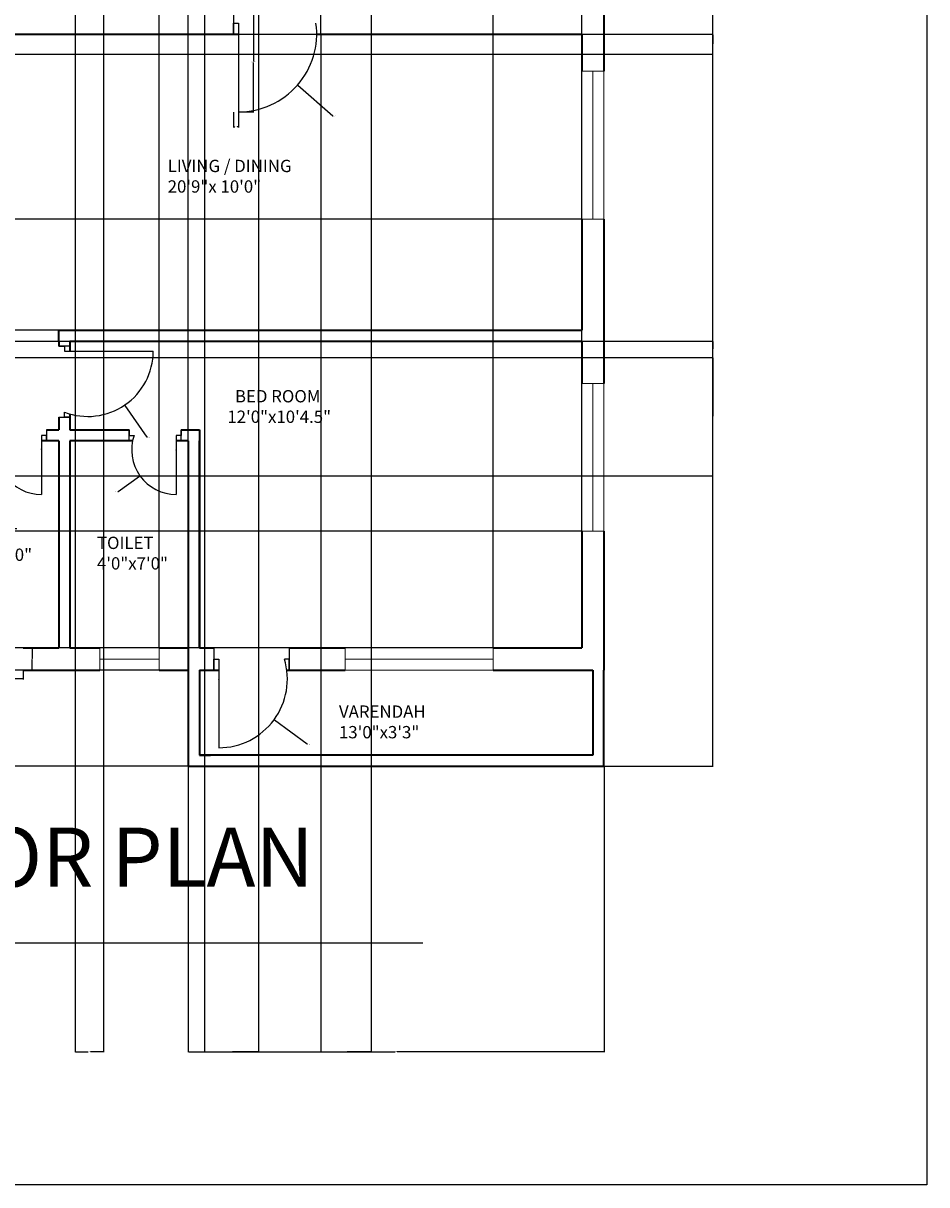
# Model space of a CAD drawing. Units: inches. Extents: x 1870 to 2611, y 1432 to 2511.
# Tile 2 of 5: x 2245 to 2611, y 1432 to 1903. Entities that reach past the tile are written whole.
import ezdxf

# ---------------------------------------------------------------- set-up
doc = ezdxf.new("R2010")
doc.units = ezdxf.units.IN
for name, color, linetype, lineweight in [('A-ANNO-DIMS', 2, 'Continuous', 18), ('A-ANNO-TTLB', 7, 'Continuous', 25), ('A-AREA-IDEN', 7, 'Continuous', 18), ('A-DOOR', 31, 'Continuous', 25), ('A-GLAZ', 201, 'Continuous', 18), ('A-WALL', 7, 'Continuous', 35)]:
    doc.layers.add(name, color=color, linetype=linetype, lineweight=lineweight)
doc.styles.get("Standard").update_dxf_attribs({"font": 'arial.ttf'})
doc.dimstyles.get("Standard").update_dxf_attribs({"dimtxt": 0.18, "dimasz": 0.18, "dimexe": 0.18, "dimexo": 0.0625, "dimgap": 0.09, "dimtad": 0, "dimtih": 1, "dimtoh": 1, "dimdec": 4, "dimzin": 0, "dimdsep": 46, "dimtxsty": 'Standard', "dimcen": 0.09, "dimadec": 0, "dimazin": 0, "dimtfac": 1, "dimtdec": 4, "dimtofl": 0, "dimtmove": 0, "dimatfit": 3, "dimfxl": 1, "dimtolj": 1, "dimtzin": 0, "dimarcsym": 0})

# ---------------------------------------------------------------- blocks, each defined once
blk = doc.blocks.new('DOOR-LEAF-36-JAMB-4P5')
for p, q in [((36, 2), (0, 2)), ((33.75, 0), (38.25, 0)), ((36, 0), (36, 2)), ((38.25, 0), (36, 0))]:
    blk.add_line(p, q)
blk = doc.blocks.new('DOOR-LEAF-24-JAMB-4P5')
for p, q in [((2, 2.25), (2, 26.25)), ((0, 4.5), (0, 0)), ((0, 0), (0, 2.25)), ((0, 2.25), (2, 2.25))]:
    blk.add_line(p, q)
blk = doc.blocks.new('DOOR-LEAF-36-JAMB-9-B')
for p, q in [((0, 40.5), (0, 31.5)), ((0, 31.5), (0, 36)), ((0, 36), (2, 36)), ((2, 36), (2, 0))]:
    blk.add_line(p, q)
blk = doc.blocks.new('WIN-60-FRAME-9')
for p, q in [((0, 9), (0, 0)), ((60, 9), (0, 9)), ((60, 4.5), (60, 9)), ((60, 9), (60, 0)), ((0, 0), (0, 4.5)), ((0, 4.5), (60, 4.5)), ((0, 0), (60, 0))]:
    blk.add_line(p, q)
blk = doc.blocks.new('WIN-24-FRAME-9')
for p, q in [((0, 9), (0, 0)), ((24, 9), (0, 9)), ((24, 4.5), (24, 9)), ((24, 9), (24, 0)), ((0, 0), (0, 4.5)), ((0, 4.5), (24, 4.5)), ((0, 0), (24, 0))]:
    blk.add_line(p, q)
blk = doc.blocks.new('*D17')
at = {"layer": 'A-ANNO-DIMS', "color": 0, "lineweight": -2, "transparency": 16777216}
for p, q in [((2220.56, 1640.3), (2220.56, 1636.59)), ((2244.56, 1640.3), (2244.56, 1636.59)), ((2220.74, 1636.77), (2231.8, 1636.77)), ((2244.38, 1636.77), (2233.31, 1636.77))]:
    blk.add_line(p, q, dxfattribs=at)
at = {"layer": 'A-ANNO-DIMS', "color": 0, "transparency": 16777216}
for points in [[(2220.74, 1636.8), (2220.74, 1636.74), (2220.56, 1636.77)], [(2244.38, 1636.8), (2244.38, 1636.74), (2244.56, 1636.77)]]:
    blk.add_solid(points, dxfattribs=at)
at = {"layer": 'Defpoints', "color": 0, "transparency": 16777216}
for p in [(2220.56, 1640.37), (2244.56, 1640.37), (2220.56, 1636.77)]:
    blk.add_point(p, dxfattribs=at)
at = {"layer": 'A-ANNO-DIMS', "color": 0, "transparency": 16777216, "insert": (2232.56, 1636.77), "char_height": 0.18, "attachment_point": 5}
blk.add_mtext('\\A1;W3 24 TYP.', dxfattribs=at)
blk = doc.blocks.new('*D18')
at = {"layer": 'A-ANNO-DIMS', "color": 0, "lineweight": -2, "transparency": 16777216}
for p, q in [((2244.62, 1649.37), (2248.34, 1649.37)), ((2248.16, 1649.19), (2248.16, 1645.05)), ((2244.62, 1640.37), (2248.34, 1640.37)), ((2248.16, 1640.55), (2248.16, 1644.69))]:
    blk.add_line(p, q, dxfattribs=at)
at = {"layer": 'A-ANNO-DIMS', "color": 0, "transparency": 16777216}
for points in [[(2248.13, 1649.19), (2248.19, 1649.19), (2248.16, 1649.37)], [(2248.13, 1640.55), (2248.19, 1640.55), (2248.16, 1640.37)]]:
    blk.add_solid(points, dxfattribs=at)
at = {"layer": 'Defpoints', "color": 0, "transparency": 16777216}
for p in [(2244.56, 1649.37), (2244.56, 1640.37), (2248.16, 1640.37)]:
    blk.add_point(p, dxfattribs=at)
at = {"layer": 'A-ANNO-DIMS', "color": 0, "transparency": 16777216, "insert": (2248.16, 1644.87), "char_height": 0.18, "attachment_point": 5}
blk.add_mtext('\\A1;9 TYP.', dxfattribs=at)
blk = doc.blocks.new('*D21')
at = {"layer": 'A-ANNO-DIMS', "color": 0, "lineweight": -2, "transparency": 16777216}
for p, q in [((2331.96, 1907.37), (2338.15, 1907.37)), ((2337.97, 1907.19), (2337.97, 1887.3)), ((2337.97, 1867.05), (2337.97, 1886.93)), ((2331.96, 1866.87), (2338.15, 1866.87))]:
    blk.add_line(p, q, dxfattribs=at)
at = {"layer": 'A-ANNO-DIMS', "color": 0, "transparency": 16777216}
for points in [[(2337.94, 1907.19), (2338, 1907.19), (2337.97, 1907.37)], [(2337.94, 1867.05), (2338, 1867.05), (2337.97, 1866.87)]]:
    blk.add_solid(points, dxfattribs=at)
at = {"layer": 'Defpoints', "color": 0, "transparency": 16777216}
for p in [(2331.9, 1907.37), (2337.97, 1907.37), (2331.9, 1866.87)]:
    blk.add_point(p, dxfattribs=at)
at = {"layer": 'A-ANNO-DIMS', "color": 0, "transparency": 16777216, "insert": (2337.97, 1887.12), "char_height": 0.18, "attachment_point": 5}
blk.add_mtext('\\A1;DOOR D 41 TYP.', dxfattribs=at)
blk = doc.blocks.new('*D22')
at = {"layer": 'A-ANNO-DIMS', "color": 0, "lineweight": -2, "transparency": 16777216}
for p, q in [((2329.9, 1866.8), (2329.9, 1860.61)), ((2331.9, 1866.8), (2331.9, 1860.61)), ((2330.08, 1860.79), (2330.44, 1860.79)), ((2331.72, 1860.79), (2331.36, 1860.79))]:
    blk.add_line(p, q, dxfattribs=at)
at = {"layer": 'A-ANNO-DIMS', "color": 0, "transparency": 16777216}
for points in [[(2330.08, 1860.82), (2330.08, 1860.76), (2329.9, 1860.79)], [(2331.72, 1860.82), (2331.72, 1860.76), (2331.9, 1860.79)]]:
    blk.add_solid(points, dxfattribs=at)
at = {"layer": 'Defpoints', "color": 0, "transparency": 16777216}
for p in [(2329.9, 1866.87), (2331.9, 1866.87), (2331.9, 1860.79)]:
    blk.add_point(p, dxfattribs=at)
at = {"layer": 'A-ANNO-DIMS', "color": 0, "transparency": 16777216, "insert": (2330.9, 1860.79), "char_height": 0.18, "attachment_point": 5}
blk.add_mtext('\\A1;2 TYP.', dxfattribs=at)
blk = doc.blocks.new('*D26')
at = {"layer": 'A-ANNO-DIMS', "color": 0, "lineweight": -2, "transparency": 16777216}
for p, q in [((2480.2, 2405.37), (2524.47, 2405.37)), ((2524.29, 2405.19), (2524.29, 2003.55)), ((2524.29, 1601.55), (2524.29, 2003.19)), ((2480.2, 1601.37), (2524.47, 1601.37))]:
    blk.add_line(p, q, dxfattribs=at)
at = {"layer": 'A-ANNO-DIMS', "color": 0, "transparency": 16777216}
for points in [[(2524.26, 2405.19), (2524.32, 2405.19), (2524.29, 2405.37)], [(2524.26, 1601.55), (2524.32, 1601.55), (2524.29, 1601.37)]]:
    blk.add_solid(points, dxfattribs=at)
at = {"layer": 'Defpoints', "color": 0, "transparency": 16777216}
for p in [(2480.14, 2405.37), (2480.14, 1601.37), (2524.29, 1601.37)]:
    blk.add_point(p, dxfattribs=at)
at = {"layer": 'A-ANNO-DIMS', "color": 0, "transparency": 16777216, "insert": (2524.29, 2003.37), "char_height": 0.18, "attachment_point": 5}
blk.add_mtext('\\A1;804', dxfattribs=at)
blk = doc.blocks.new('*D31')
at = {"layer": 'A-ANNO-DIMS', "color": 0, "lineweight": -2, "transparency": 16777216}
for p, q in [((2311.52, 1601.3), (2311.52, 1485.35)), ((2480.14, 1601.3), (2480.14, 1485.35)), ((2311.7, 1485.53), (2395.37, 1485.53)), ((2479.96, 1485.53), (2396.28, 1485.53))]:
    blk.add_line(p, q, dxfattribs=at)
at = {"layer": 'A-ANNO-DIMS', "color": 0, "transparency": 16777216}
for points in [[(2311.7, 1485.56), (2311.7, 1485.5), (2311.52, 1485.53)], [(2479.96, 1485.56), (2479.96, 1485.5), (2480.14, 1485.53)]]:
    blk.add_solid(points, dxfattribs=at)
at = {"layer": 'Defpoints', "color": 0, "transparency": 16777216}
for p in [(2311.52, 1601.36), (2480.14, 1601.37), (2480.14, 1485.53)]:
    blk.add_point(p, dxfattribs=at)
at = {"layer": 'A-ANNO-DIMS', "color": 0, "transparency": 16777216, "insert": (2395.83, 1485.53), "char_height": 0.18, "attachment_point": 5}
blk.add_mtext('\\A1;168.62', dxfattribs=at)
blk = doc.blocks.new('*D32')
at = {"layer": 'A-ANNO-DIMS', "color": 0, "lineweight": -2, "transparency": 16777216}
for p, q in [((2311.46, 1640.37), (1960.31, 1640.37)), ((1960.49, 1640.19), (1960.49, 1621.05)), ((1960.49, 1601.54), (1960.49, 1620.68)), ((2311.46, 1601.36), (1960.31, 1601.36))]:
    blk.add_line(p, q, dxfattribs=at)
at = {"layer": 'A-ANNO-DIMS', "color": 0, "transparency": 16777216}
for points in [[(1960.46, 1640.19), (1960.52, 1640.19), (1960.49, 1640.37)], [(1960.46, 1601.54), (1960.52, 1601.54), (1960.49, 1601.36)]]:
    blk.add_solid(points, dxfattribs=at)
at = {"layer": 'Defpoints', "color": 0, "transparency": 16777216}
for p in [(1960.49, 1640.37), (2311.52, 1640.37), (2311.52, 1601.36)]:
    blk.add_point(p, dxfattribs=at)
at = {"layer": 'A-ANNO-DIMS', "color": 0, "transparency": 16777216, "insert": (1960.49, 1620.86), "char_height": 0.18, "attachment_point": 5}
blk.add_mtext('\\A1;39.01', dxfattribs=at)
blk = doc.blocks.new('*D38')
at = {"layer": 'A-ANNO-DIMS', "color": 0, "lineweight": -2, "transparency": 16777216}
for p, q in [((2385.64, 1907.3), (2385.64, 1485.35)), ((2365.31, 1898.3), (2365.31, 1485.35)), ((2365.49, 1485.53), (2375.01, 1485.53)), ((2385.46, 1485.53), (2375.94, 1485.53))]:
    blk.add_line(p, q, dxfattribs=at)
at = {"layer": 'A-ANNO-DIMS', "color": 0, "transparency": 16777216}
for points in [[(2365.49, 1485.56), (2365.49, 1485.5), (2365.31, 1485.53)], [(2385.46, 1485.56), (2385.46, 1485.5), (2385.64, 1485.53)]]:
    blk.add_solid(points, dxfattribs=at)
at = {"layer": 'Defpoints', "color": 0, "transparency": 16777216}
for p in [(2385.64, 1907.37), (2365.31, 1898.37), (2385.64, 1485.53)]:
    blk.add_point(p, dxfattribs=at)
at = {"layer": 'A-ANNO-DIMS', "color": 0, "transparency": 16777216, "insert": (2375.47, 1485.53), "char_height": 0.18, "attachment_point": 5}
blk.add_mtext('\\A1;20.328', dxfattribs=at)
blk = doc.blocks.new('*D41')
at = {"layer": 'A-ANNO-DIMS', "color": 0, "lineweight": -2, "transparency": 16777216}
for p, q in [((2265.64, 2396.3), (2265.64, 1485.35)), ((2277.17, 2396.3), (2277.17, 1485.35)), ((2265.82, 1485.53), (2270.95, 1485.53)), ((2276.99, 1485.53), (2271.86, 1485.53))]:
    blk.add_line(p, q, dxfattribs=at)
at = {"layer": 'A-ANNO-DIMS', "color": 0, "transparency": 16777216}
for points in [[(2265.82, 1485.56), (2265.82, 1485.5), (2265.64, 1485.53)], [(2276.99, 1485.56), (2276.99, 1485.5), (2277.17, 1485.53)]]:
    blk.add_solid(points, dxfattribs=at)
at = {"layer": 'Defpoints', "color": 0, "transparency": 16777216}
for p in [(2265.64, 2396.37), (2277.17, 2396.37), (2277.17, 1485.53)]:
    blk.add_point(p, dxfattribs=at)
at = {"layer": 'A-ANNO-DIMS', "color": 0, "transparency": 16777216, "insert": (2271.4, 1485.53), "char_height": 0.18, "attachment_point": 5}
blk.add_mtext('\\A1;11.535', dxfattribs=at)
blk = doc.blocks.new('*D42')
at = {"layer": 'A-ANNO-DIMS', "color": 0, "lineweight": -2, "transparency": 16777216}
for p, q in [((2318.14, 2396.3), (2318.14, 1485.35)), ((2340.04, 2396.3), (2340.04, 1485.35)), ((2318.32, 1485.53), (2328.76, 1485.53)), ((2339.86, 1485.53), (2329.41, 1485.53))]:
    blk.add_line(p, q, dxfattribs=at)
at = {"layer": 'A-ANNO-DIMS', "color": 0, "transparency": 16777216}
for points in [[(2318.32, 1485.56), (2318.32, 1485.5), (2318.14, 1485.53)], [(2339.86, 1485.56), (2339.86, 1485.5), (2340.04, 1485.53)]]:
    blk.add_solid(points, dxfattribs=at)
at = {"layer": 'Defpoints', "color": 0, "transparency": 16777216}
for p in [(2318.14, 2396.37), (2340.04, 2396.37), (2340.04, 1485.53)]:
    blk.add_point(p, dxfattribs=at)
at = {"layer": 'A-ANNO-DIMS', "color": 0, "transparency": 16777216, "insert": (2329.09, 1485.53), "char_height": 0.18, "attachment_point": 5}
blk.add_mtext('\\A1;21.9', dxfattribs=at)
blk = doc.blocks.new('*D46')
at = {"layer": 'A-ANNO-DIMS', "color": 0, "lineweight": -2, "transparency": 16777216}
for p, q in [((2299.67, 1649.43), (2299.67, 2449.7)), ((2299.85, 2449.52), (2305.14, 2449.52)), ((2311.34, 2449.52), (2306.05, 2449.52)), ((2311.52, 1649.43), (2311.52, 2449.7))]:
    blk.add_line(p, q, dxfattribs=at)
at = {"layer": 'A-ANNO-DIMS', "color": 0, "transparency": 16777216}
for points in [[(2299.85, 2449.55), (2299.85, 2449.49), (2299.67, 2449.52)], [(2311.34, 2449.55), (2311.34, 2449.49), (2311.52, 2449.52)]]:
    blk.add_solid(points, dxfattribs=at)
at = {"layer": 'Defpoints', "color": 0, "transparency": 16777216}
for p in [(2311.52, 2449.52), (2299.67, 1649.37), (2311.52, 1649.37)]:
    blk.add_point(p, dxfattribs=at)
at = {"layer": 'A-ANNO-DIMS', "color": 0, "transparency": 16777216, "insert": (2305.6, 2449.52), "char_height": 0.18, "attachment_point": 5}
blk.add_mtext('\\A1;11.846', dxfattribs=at)
blk = doc.blocks.new('*D47')
at = {"layer": 'A-ANNO-DIMS', "color": 0, "lineweight": -2, "transparency": 16777216}
for p, q in [((2435.2, 1649.43), (2435.2, 2449.7)), ((2435.38, 2449.52), (2452.77, 2449.52)), ((2470.96, 2449.52), (2453.56, 2449.52)), ((2471.14, 1649.43), (2471.14, 2449.7))]:
    blk.add_line(p, q, dxfattribs=at)
at = {"layer": 'A-ANNO-DIMS', "color": 0, "transparency": 16777216}
for points in [[(2435.38, 2449.55), (2435.38, 2449.49), (2435.2, 2449.52)], [(2470.96, 2449.55), (2470.96, 2449.49), (2471.14, 2449.52)]]:
    blk.add_solid(points, dxfattribs=at)
at = {"layer": 'Defpoints', "color": 0, "transparency": 16777216}
for p in [(2471.14, 2449.52), (2435.2, 1649.37), (2471.14, 1649.37)]:
    blk.add_point(p, dxfattribs=at)
at = {"layer": 'A-ANNO-DIMS', "color": 0, "transparency": 16777216, "insert": (2453.17, 2449.52), "char_height": 0.18, "attachment_point": 5}
blk.add_mtext('\\A1;35.94', dxfattribs=at)
blk = doc.blocks.new('*D49')
at = {"layer": 'A-ANNO-DIMS', "color": 0, "lineweight": -2, "transparency": 16777216}
for p, q in [((2471.07, 1823.42), (1960.31, 1823.42)), ((1960.49, 1823.24), (1960.49, 1801.08)), ((1960.49, 1778.55), (1960.49, 1800.71)), ((2471.07, 1778.37), (1960.31, 1778.37))]:
    blk.add_line(p, q, dxfattribs=at)
at = {"layer": 'A-ANNO-DIMS', "color": 0, "transparency": 16777216}
for points in [[(1960.46, 1823.24), (1960.52, 1823.24), (1960.49, 1823.42)], [(1960.46, 1778.55), (1960.52, 1778.55), (1960.49, 1778.37)]]:
    blk.add_solid(points, dxfattribs=at)
at = {"layer": 'Defpoints', "color": 0, "transparency": 16777216}
for p in [(1960.49, 1823.42), (2471.14, 1823.42), (2471.14, 1778.37)]:
    blk.add_point(p, dxfattribs=at)
at = {"layer": 'A-ANNO-DIMS', "color": 0, "transparency": 16777216, "insert": (1960.49, 1800.89), "char_height": 0.18, "attachment_point": 5}
blk.add_mtext('\\A1;45.05', dxfattribs=at)
blk = doc.blocks.new('*D50')
at = {"layer": 'A-ANNO-DIMS', "color": 0, "lineweight": -2, "transparency": 16777216}
for p, q in [((2471.07, 1696.72), (1960.31, 1696.72)), ((1960.49, 1696.54), (1960.49, 1673.22)), ((1960.49, 1649.55), (1960.49, 1672.86)), ((2471.07, 1649.37), (1960.31, 1649.37))]:
    blk.add_line(p, q, dxfattribs=at)
at = {"layer": 'A-ANNO-DIMS', "color": 0, "transparency": 16777216}
for points in [[(1960.46, 1696.54), (1960.52, 1696.54), (1960.49, 1696.72)], [(1960.46, 1649.55), (1960.52, 1649.55), (1960.49, 1649.37)]]:
    blk.add_solid(points, dxfattribs=at)
at = {"layer": 'Defpoints', "color": 0, "transparency": 16777216}
for p in [(1960.49, 1696.72), (2471.14, 1696.72), (2471.14, 1649.37)]:
    blk.add_point(p, dxfattribs=at)
at = {"layer": 'A-ANNO-DIMS', "color": 0, "transparency": 16777216, "insert": (1960.49, 1673.04), "char_height": 0.18, "attachment_point": 5}
blk.add_mtext('\\A1;47.35', dxfattribs=at)
blk = doc.blocks.new('*D55')
at = {"layer": 'A-ANNO-DIMS', "color": 0, "lineweight": -2, "transparency": 16777216}
for p, q in [((2074.58, 1898.37), (2524.47, 1898.37)), ((2524.29, 1898.19), (2524.29, 1894.51)), ((2074.58, 1890.28), (2524.47, 1890.28)), ((2524.29, 1890.46), (2524.29, 1894.14))]:
    blk.add_line(p, q, dxfattribs=at)
at = {"layer": 'A-ANNO-DIMS', "color": 0, "transparency": 16777216}
for points in [[(2524.26, 1898.19), (2524.32, 1898.19), (2524.29, 1898.37)], [(2524.26, 1890.46), (2524.32, 1890.46), (2524.29, 1890.28)]]:
    blk.add_solid(points, dxfattribs=at)
at = {"layer": 'Defpoints', "color": 0, "transparency": 16777216}
for p in [(2074.52, 1898.37), (2524.29, 1898.37), (2074.52, 1890.28)]:
    blk.add_point(p, dxfattribs=at)
at = {"layer": 'A-ANNO-DIMS', "color": 0, "transparency": 16777216, "insert": (2524.29, 1894.32), "char_height": 0.18, "attachment_point": 5}
blk.add_mtext('\\A1;8.085', dxfattribs=at)
blk = doc.blocks.new('*D56')
at = {"layer": 'A-ANNO-DIMS', "color": 0, "lineweight": -2, "transparency": 16777216}
for p, q in [((2074.58, 1767.26), (2524.47, 1767.26)), ((2524.29, 1767.08), (2524.29, 1743.44)), ((2524.29, 1719.44), (2524.29, 1743.08)), ((2074.58, 1719.26), (2524.47, 1719.26))]:
    blk.add_line(p, q, dxfattribs=at)
at = {"layer": 'A-ANNO-DIMS', "color": 0, "transparency": 16777216}
for points in [[(2524.26, 1767.08), (2524.32, 1767.08), (2524.29, 1767.26)], [(2524.26, 1719.44), (2524.32, 1719.44), (2524.29, 1719.26)]]:
    blk.add_solid(points, dxfattribs=at)
at = {"layer": 'Defpoints', "color": 0, "transparency": 16777216}
for p in [(2074.52, 1767.26), (2524.29, 1767.26), (2074.52, 1719.26)]:
    blk.add_point(p, dxfattribs=at)
at = {"layer": 'A-ANNO-DIMS', "color": 0, "transparency": 16777216, "insert": (2524.29, 1743.26), "char_height": 0.18, "attachment_point": 5}
blk.add_mtext('\\A1;48', dxfattribs=at)
blk = doc.blocks.new('*D57')
at = {"layer": 'A-ANNO-DIMS', "color": 0, "lineweight": -2, "transparency": 16777216}
for p, q in [((2074.58, 1773.87), (2524.47, 1773.87)), ((2524.29, 1773.69), (2524.29, 1770.74)), ((2524.29, 1767.44), (2524.29, 1770.38)), ((2074.58, 1767.26), (2524.47, 1767.26))]:
    blk.add_line(p, q, dxfattribs=at)
at = {"layer": 'A-ANNO-DIMS', "color": 0, "transparency": 16777216}
for points in [[(2524.26, 1773.69), (2524.32, 1773.69), (2524.29, 1773.87)], [(2524.26, 1767.44), (2524.32, 1767.44), (2524.29, 1767.26)]]:
    blk.add_solid(points, dxfattribs=at)
at = {"layer": 'Defpoints', "color": 0, "transparency": 16777216}
for p in [(2074.52, 1773.87), (2524.29, 1773.87), (2074.52, 1767.26)]:
    blk.add_point(p, dxfattribs=at)
at = {"layer": 'A-ANNO-DIMS', "color": 0, "transparency": 16777216, "insert": (2524.29, 1770.56), "char_height": 0.18, "attachment_point": 5}
blk.add_mtext('\\A1;6.61', dxfattribs=at)
blk = doc.blocks.new('*D59')
at = {"layer": 'A-ANNO-DIMS', "color": 0, "lineweight": -2, "transparency": 16777216}
for p, q in [((2331.81, 1898.57), (2331.99, 1898.57)), ((2331.9, 1898.48), (2331.9, 1898.66)), ((2370.12, 1865.22), (2355.92, 1877.61)), ((2370.3, 1865.22), (2370.12, 1865.22))]:
    blk.add_line(p, q, dxfattribs=at)
at = {"layer": 'A-ANNO-DIMS', "color": 0, "transparency": 16777216}
blk.add_solid([(2355.94, 1877.63), (2355.9, 1877.59), (2355.79, 1877.73)], dxfattribs=at)
at = {"layer": 'Defpoints', "color": 0, "transparency": 16777216}
for p in [(2331.9, 1898.57), (2355.79, 1877.73)]:
    blk.add_point(p, dxfattribs=at)
at = {"layer": 'A-ANNO-DIMS', "color": 0, "transparency": 16777216, "insert": (2370.85, 1865.22), "char_height": 0.18, "attachment_point": 5}
blk.add_mtext('\\A1;R31.704', dxfattribs=at)
blk = doc.blocks.new('*D64')
at = {"layer": 'A-ANNO-DIMS', "color": 0, "lineweight": -2, "transparency": 16777216}
for p, q in [((2323.82, 1636.66), (2324, 1636.66)), ((2323.91, 1636.57), (2323.91, 1636.75)), ((2359.7, 1610.26), (2346.42, 1620.06)), ((2359.88, 1610.26), (2359.7, 1610.26))]:
    blk.add_line(p, q, dxfattribs=at)
at = {"layer": 'A-ANNO-DIMS', "color": 0, "transparency": 16777216}
blk.add_solid([(2346.44, 1620.08), (2346.41, 1620.03), (2346.28, 1620.16)], dxfattribs=at)
at = {"layer": 'Defpoints', "color": 0, "transparency": 16777216}
for p in [(2323.91, 1636.66), (2346.28, 1620.16)]:
    blk.add_point(p, dxfattribs=at)
at = {"layer": 'A-ANNO-DIMS', "color": 0, "transparency": 16777216, "insert": (2360.43, 1610.26), "char_height": 0.18, "attachment_point": 5}
blk.add_mtext('\\A1;R27.796', dxfattribs=at)
blk = doc.blocks.new('*D66')
at = {"layer": 'A-ANNO-DIMS', "color": 0, "lineweight": -2, "transparency": 16777216}
for p, q in [((2270.69, 1769.79), (2270.87, 1769.79)), ((2270.78, 1769.7), (2270.78, 1769.88)), ((2294.77, 1734.86), (2285.88, 1747.81)), ((2294.95, 1734.86), (2294.77, 1734.86))]:
    blk.add_line(p, q, dxfattribs=at)
at = {"layer": 'A-ANNO-DIMS', "color": 0, "transparency": 16777216}
blk.add_solid([(2285.9, 1747.83), (2285.85, 1747.79), (2285.77, 1747.96)], dxfattribs=at)
at = {"layer": 'Defpoints', "color": 0, "transparency": 16777216}
for p in [(2270.78, 1769.79), (2285.77, 1747.96)]:
    blk.add_point(p, dxfattribs=at)
at = {"layer": 'A-ANNO-DIMS', "color": 0, "transparency": 16777216, "insert": (2295.5, 1734.86), "char_height": 0.18, "attachment_point": 5}
blk.add_mtext('\\A1;R26.484', dxfattribs=at)
blk = doc.blocks.new('*D74')
at = {"layer": 'A-ANNO-DIMS', "color": 0, "lineweight": -2, "transparency": 16777216}
for p, q in [((2251.93, 1730.01), (2252.11, 1730.01)), ((2252.02, 1729.92), (2252.02, 1730.1)), ((2228.25, 1712.66), (2237.02, 1719.06)), ((2228.07, 1712.66), (2228.25, 1712.66))]:
    blk.add_line(p, q, dxfattribs=at)
at = {"layer": 'A-ANNO-DIMS', "color": 0, "transparency": 16777216}
blk.add_solid([(2237, 1719.08), (2237.04, 1719.04), (2237.17, 1719.17)], dxfattribs=at)
at = {"layer": 'Defpoints', "color": 0, "transparency": 16777216}
for p in [(2252.02, 1730.01), (2237.17, 1719.17)]:
    blk.add_point(p, dxfattribs=at)
at = {"layer": 'A-ANNO-DIMS', "color": 0, "transparency": 16777216, "insert": (2227.59, 1712.66), "char_height": 0.18, "attachment_point": 5}
blk.add_mtext('\\A1;R18.39', dxfattribs=at)
blk = doc.blocks.new('*D76')
at = {"layer": 'A-ANNO-DIMS', "color": 0, "lineweight": -2, "transparency": 16777216}
for p, q in [((2306.65, 1729.64), (2306.65, 1729.82)), ((2306.56, 1729.73), (2306.74, 1729.73)), ((2283.06, 1712.89), (2291.76, 1719.1)), ((2282.88, 1712.89), (2283.06, 1712.89))]:
    blk.add_line(p, q, dxfattribs=at)
at = {"layer": 'A-ANNO-DIMS', "color": 0, "transparency": 16777216}
blk.add_solid([(2291.74, 1719.13), (2291.78, 1719.08), (2291.91, 1719.21)], dxfattribs=at)
at = {"layer": 'Defpoints', "color": 0, "transparency": 16777216}
for p in [(2306.65, 1729.73), (2291.91, 1719.21)]:
    blk.add_point(p, dxfattribs=at)
at = {"layer": 'A-ANNO-DIMS', "color": 0, "transparency": 16777216, "insert": (2282.33, 1712.89), "char_height": 0.18, "attachment_point": 5}
blk.add_mtext('\\A1;R18.114', dxfattribs=at)

msp = doc.modelspace()

# ---------------------------------------------------------------- linework, layer by layer
at = {"layer": 'A-ANNO-TTLB'}
for p in [(2050.9784, 1529.6813), (2406.6559, 1529.6813)]:
    msp.add_line(p, (2406.6559, 1529.6813), dxfattribs=at)
msp.add_lwpolyline([(1869.7418, 2510.8018), (2611.0646, 2510.8018), (2611.0646, 1431.531), (1869.7418, 1431.531)], close=True, dxfattribs=at)
at = {"layer": 'A-DOOR'}
for p, q in [((2365.3084, 1898.3669), (2365.3084, 1907.3669)), ((2261.2682, 1743.0751), (2261.2682, 1745.0751)), ((2259.0182, 1743.0751), (2263.5182, 1743.0751)), ((2263.5182, 1743.0751), (2261.2682, 1743.0751)), ((2254.0217, 1735.6169), (2252.0217, 1735.6169)), ((2252.0217, 1735.6169), (2252.0217, 1711.6169)), ((2254.0217, 1737.8669), (2254.0217, 1733.3669)), ((2254.0217, 1733.3669), (2254.0217, 1735.6169)), ((2287.5182, 1733.3669), (2287.5182, 1737.8669)), ((2287.5182, 1737.8669), (2287.5182, 1735.6169)), ((2287.5182, 1735.6169), (2289.5182, 1735.6169)), ((2254.0217, 1733.3669), (2254.0217, 1733.3669)), ((2352.4679, 1649.3669), (2352.4679, 1640.3669)), ((2321.9097, 1644.8669), (2321.9097, 1644.8669)), ((2352.4679, 1644.8669), (2350.4679, 1644.8669)), ((2352.4679, 1640.3669), (2352.4679, 1644.8669))]:
    msp.add_line(p, q, dxfattribs=at)
for centre, radius, start, end in [((2331.8969, 1898.5708), 31.7039, 270, 7.788013), ((2270.7841, 1769.7906), 26.4841, 248.942434, 0), ((2252.0217, 1730.0064), 18.3894, 162.235951, 270), ((2306.6497, 1729.7312), 18.1143, 161.039319, 270), ((2323.9097, 1636.6633), 27.7964, 270, 17.165418)]:
    msp.add_arc(centre, radius, start, end, dxfattribs=at)
at = {"layer": 'A-GLAZ'}
for p, q in [((2471.1359, 1883.4206), (2480.1359, 1883.4206)), ((2471.1359, 1883.4206), (2471.1359, 1823.4206)), ((2480.1359, 1883.4206), (2475.6359, 1883.4206)), ((2475.6359, 1883.4206), (2475.6359, 1835.4206)), ((2480.1359, 1883.4206), (2480.1359, 1823.4206)), ((2475.6359, 1835.4206), (2475.6359, 1823.4206)), ((2475.6359, 1823.4206), (2471.1359, 1823.4206)), ((2471.1359, 1823.4206), (2480.1359, 1823.4206)), ((2471.1359, 1756.7177), (2471.1359, 1756.7177)), ((2471.1359, 1756.7177), (2471.1359, 1756.7177)), ((2471.1359, 1756.7177), (2471.1359, 1756.7177)), ((2475.6359, 1756.7177), (2475.6359, 1756.7177)), ((2375.1985, 1644.8669), (2375.1985, 1644.8669)), ((2435.1985, 1640.3669), (2435.1985, 1640.3669))]:
    msp.add_line(p, q, dxfattribs=at)
at = {"layer": 'A-WALL'}
for p, q in [((2480.1359, 2178.5402), (2480.1359, 1883.4206)), ((2211.0182, 1898.3669), (2331.8969, 1898.3669)), ((2363.6001, 1898.3669), (2471.1359, 1898.3669)), ((2471.1359, 1898.3669), (2471.1359, 1883.4206)), ((2471.1359, 1823.4206), (2471.1359, 1778.3669)), ((2480.1359, 1823.4206), (2480.1359, 1756.7177)), ((2259.0182, 1773.8669), (2259.0182, 1778.3669)), ((2259.0182, 1778.3669), (2471.1359, 1778.3669)), ((2259.0182, 1773.8669), (2259.0182, 1771.7906)), ((2263.5182, 1773.8669), (2263.5182, 1769.7906)), ((2263.5182, 1773.8669), (2471.1359, 1773.8669)), ((2471.1359, 1773.8669), (2471.1359, 1756.7177)), ((2263.5182, 1744.3227), (2263.5182, 1737.8669)), ((2259.0182, 1743.0751), (2259.0182, 1737.8669)), ((2254.0217, 1737.8669), (2259.0182, 1737.8669)), ((2263.5182, 1737.8669), (2287.5182, 1737.8669)), ((2308.6497, 1737.8669), (2316.0182, 1737.8669)), ((2316.0182, 1737.8669), (2316.0182, 1649.3669)), ((2259.0182, 1733.3669), (2252.0217, 1733.3669)), ((2259.0182, 1733.3669), (2259.0182, 1649.3669)), ((2263.5182, 1733.3669), (2263.5182, 1649.3669)), ((2288.904, 1733.3669), (2263.5182, 1733.3669)), ((2311.5182, 1733.3669), (2306.6497, 1733.3669)), ((2311.5182, 1733.3669), (2311.5182, 1649.3669)), ((2316.0182, 1649.3669), (2316.0182, 1733.3669)), ((2471.1359, 1696.7177), (2471.1359, 1649.3669)), ((2480.1359, 1696.7177), (2480.1359, 1640.3669)), ((2316.0182, 1651.6374), (2316.0182, 1649.3669)), ((2244.5557, 1649.3669), (2259.0182, 1649.3669)), ((2263.5182, 1649.3669), (2275.6725, 1649.3669)), ((2299.6725, 1649.3669), (2311.5182, 1649.3669)), ((2311.5182, 1649.3669), (2311.5182, 1601.3597)), ((2316.0182, 1649.3669), (2321.9097, 1649.3669)), ((2352.4679, 1649.3669), (2375.1985, 1649.3669)), ((2435.1985, 1649.3669), (2471.1359, 1649.3669)), ((2244.5557, 1640.3669), (2275.6725, 1640.3669)), ((2299.6725, 1640.3669), (2311.5182, 1640.3669)), ((2316.0182, 1640.3669), (2316.0182, 1605.8669)), ((2316.0182, 1640.3669), (2323.9097, 1640.3669)), ((2351.4582, 1640.3669), (2375.1985, 1640.3669)), ((2435.1985, 1640.3669), (2475.6359, 1640.3669)), ((2475.6359, 1640.3669), (2475.6359, 1605.8669)), ((2480.1359, 1601.3669), (2480.1359, 1640.3669)), ((2475.6359, 1605.8669), (2316.0182, 1605.8669)), ((2316.0182, 1605.8669), (2320.5182, 1605.8669)), ((2311.5182, 1601.3597), (2316.0182, 1601.3669)), ((2316.0182, 1601.3669), (2480.1359, 1601.3669)), ((2475.6359, 1601.3669), (2475.6359, 1601.3669))]:
    msp.add_line(p, q, dxfattribs=at)

# ---------------------------------------------------------------- block references
at = {"layer": 'A-DOOR'}
for p in [(2329.897, 1866.867), (2321.9097, 1608.867)]:
    msp.add_blockref('DOOR-LEAF-36-JAMB-9-B', p, dxfattribs=at)
at = {"layer": 'A-DOOR', "rotation": 180}
for name, p in [('DOOR-LEAF-36-JAMB-4P5', (2297.2682, 1771.7907)), ('DOOR-LEAF-24-JAMB-4P5', (2308.65, 1737.8669))]:
    msp.add_blockref(name, p, dxfattribs=at)
at = {"layer": 'A-GLAZ', "extrusion": (0, 0, -1), "zscale": -1, "rotation": 270}
msp.add_blockref('WIN-60-FRAME-9', (-2480.1359, 1756.7175), dxfattribs=at)
at = {"layer": 'A-GLAZ', "rotation": 180}
msp.add_blockref('WIN-24-FRAME-9', (2299.6723, 1649.3669), dxfattribs=at)
at = {"layer": 'A-GLAZ'}
msp.add_blockref('WIN-60-FRAME-9', (2375.1987, 1640.367), dxfattribs=at)

# ---------------------------------------------------------------- texts
at = {"layer": 'A-ANNO-TTLB', "insert": (2072.8808, 1576.4623), "char_height": 24, "attachment_point": 1}
msp.add_mtext_dynamic_manual_height_columns('FIRST FLOOR PLAN', width=470.964305, gutter_width=12.5, heights=[0], dxfattribs=at)
at = {"layer": 'A-AREA-IDEN', "char_height": 5, "attachment_point": 1}
for s, width, insert in [('LIVING / DINING\\P20\'9"x 10\'0"', 114.417189, (2303.1557, 1847.4581)), ('  BED ROOM\\P12\'0"x10\'4.5"', 143.764477, (2327.3714, 1754.0113)), ('TOILET\\P4\'0"x7\'0"', 39.670567, (2219.3477, 1698.0164)), ('TOILET\\P4\'0"x7\'0"', 33.618884, (2274.4642, 1694.513)), ('VARENDAH\\P13\'0"x3\'3"', 102.636332, (2372.6381, 1626.0203))]:
    msp.add_mtext_dynamic_manual_height_columns(s, width=width, gutter_width=12.5, heights=[0], dxfattribs=dict(at, insert=insert))

# ---------------------------------------------------------------- dimensions: what is measured, and where the dimension line sits
at = {"layer": 'A-ANNO-DIMS'}
for base, p1, p2, override, picture, middle in [((2311.5182, 2449.5169), (2299.6725, 1649.3669), (2311.5182, 1649.3669), {"dimdec": 3, "dimlfac": 1, "dimrnd": 0, "dimzin": 0, "dimdsep": 46, "dimlunit": 2}, '*D46', (2305.5954, 2449.5169)), ((2471.1359, 2449.5169), (2435.1985, 1649.3669), (2471.1359, 1649.3669), {"dimdec": 2, "dimlfac": 1, "dimrnd": 0, "dimzin": 0, "dimdsep": 46, "dimlunit": 2}, '*D47', (2453.1672, 2449.5169)), ((2277.1709, 1485.5313), (2265.6359, 2396.3669), (2277.1709, 2396.3669), {"dimdec": 3, "dimlfac": 1, "dimrnd": 0, "dimzin": 0, "dimdsep": 46, "dimlunit": 2}, '*D41', (2271.4034, 1485.5313)), ((2340.0375, 1485.5313), (2318.1359, 2396.3669), (2340.0375, 2396.3669), {"dimdec": 1, "dimlfac": 1, "dimrnd": 0, "dimzin": 0, "dimdsep": 46, "dimlunit": 2}, '*D42', (2329.0867, 1485.5313)), ((2385.63592, 1485.53127), (2365.30836, 1898.36694), (2385.63592, 1907.36694), {"dimdec": 3, "dimlfac": 1, "dimrnd": 0, "dimzin": 0, "dimdsep": 46, "dimlunit": 2}, '*D38', (2375.47214, 1485.53127)), ((2480.1359, 1485.5313), (2311.5182, 1601.3597), (2480.1359, 1601.3669), {"dimdec": 2, "dimlfac": 1, "dimrnd": 0, "dimzin": 0, "dimdsep": 46, "dimlunit": 2}, '*D31', (2395.8271, 1485.5313))]:
    dim = msp.add_linear_dim(base=base, p1=p1, p2=p2, dimstyle='Standard', override=override, dxfattribs=at)
    dim.commit()
    dim.dimension.update_dxf_attribs({"geometry": picture, "text_midpoint": middle})
for base, p1, p2, override, picture, middle in [((2524.2859, 1601.3669), (2480.1359, 2405.3669), (2480.1359, 1601.3669), {"dimdec": 0, "dimlfac": 1, "dimrnd": 0, "dimzin": 0, "dimdsep": 46, "dimlunit": 2}, '*D26', (2524.2859, 2003.3669)), ((2524.2859, 1898.3669), (2074.5182, 1890.2819), (2074.5182, 1898.3669), {"dimdec": 3, "dimlfac": 1, "dimrnd": 0, "dimzin": 0, "dimdsep": 46, "dimlunit": 2}, '*D55', (2524.2859, 1894.3244)), ((1960.4859, 1823.4206), (2471.1359, 1778.3669), (2471.1359, 1823.4206), {"dimdec": 2, "dimlfac": 1, "dimrnd": 0, "dimzin": 0, "dimdsep": 46, "dimlunit": 2}, '*D49', (1960.4859, 1800.8937)), ((2524.2859, 1773.8669), (2074.5182, 1767.257), (2074.5182, 1773.8669), {"dimdec": 2, "dimlfac": 1, "dimrnd": 0, "dimzin": 0, "dimdsep": 46, "dimlunit": 2}, '*D57', (2524.2859, 1770.562)), ((2524.2859, 1767.257), (2074.5182, 1719.257), (2074.5182, 1767.257), {"dimdec": 0, "dimlfac": 1, "dimrnd": 0, "dimzin": 0, "dimdsep": 46, "dimlunit": 2}, '*D56', (2524.2859, 1743.257)), ((1960.4859, 1696.7177), (2471.1359, 1649.3669), (2471.1359, 1696.7177), {"dimdec": 2, "dimlfac": 1, "dimrnd": 0, "dimzin": 0, "dimdsep": 46, "dimlunit": 2}, '*D50', (1960.4859, 1673.0423)), ((1960.4859, 1640.3669), (2311.5182, 1601.3597), (2311.5182, 1640.3669), {"dimdec": 2, "dimlfac": 1, "dimrnd": 0, "dimzin": 0, "dimdsep": 46, "dimlunit": 2}, '*D32', (1960.4859, 1620.8633))]:
    dim = msp.add_linear_dim(base=base, p1=p1, p2=p2, angle=90, dimstyle='Standard', override=override, dxfattribs=at)
    dim.commit()
    dim.dimension.update_dxf_attribs({"geometry": picture, "text_midpoint": middle})
for base, p1, p2, angle, text, picture, middle in [((2337.9719273778, 1907.3669377198), (2331.8969273778, 1866.8669377198), (2331.8969273778, 1907.3669377198), 90, 'DOOR D <> TYP.', '*D21', (2337.9719273778, 1887.1169377198)), ((2248.1557, 1640.3669), (2244.5557, 1649.3669), (2244.5557, 1640.3669), 270, '<> TYP.', '*D18', (2248.1557, 1644.8669)), ((2220.5557, 1636.7669), (2244.5557, 1640.3669), (2220.5557, 1640.3669), 180, 'W3 <> TYP.', '*D17', (2232.5557, 1636.7669))]:
    dim = msp.add_linear_dim(base=base, p1=p1, p2=p2, angle=angle, text=text, dimstyle='Standard', override={"dimdec": 0, "dimlfac": 1, "dimrnd": 0, "dimzin": 0, "dimdsep": 46, "dimlunit": 2}, dxfattribs=at)
    dim.commit()
    dim.dimension.update_dxf_attribs({"geometry": picture, "text_midpoint": middle})
for center, mpoint, override, picture, middle in [((2331.8969, 1898.5708), (2355.7858, 1877.7272), {"dimdec": 3, "dimlfac": 1, "dimrnd": 0, "dimzin": 0, "dimdsep": 46, "dimlunit": 2}, '*D59', (2370.8485, 1865.221)), ((2270.7841, 1769.7906), (2285.774, 1747.9569), {"dimdec": 3, "dimlfac": 1, "dimrnd": 0, "dimzin": 0, "dimdsep": 46, "dimlunit": 2}, '*D66', (2295.4974, 1734.8567)), ((2252.0217, 1730.0064), (2237.1666, 1719.1667), {"dimdec": 2, "dimlfac": 1, "dimrnd": 0, "dimzin": 0, "dimdsep": 46, "dimlunit": 2}, '*D74', (2227.5936, 1712.663)), ((2306.6497, 1729.7312), (2291.9062, 1719.2071), {"dimdec": 3, "dimlfac": 1, "dimrnd": 0, "dimzin": 0, "dimdsep": 46, "dimlunit": 2}, '*D76', (2282.3307, 1712.8927)), ((2323.9097, 1636.6633), (2346.278, 1620.162), {"dimdec": 3, "dimlfac": 1, "dimrnd": 0, "dimzin": 0, "dimdsep": 46, "dimlunit": 2}, '*D64', (2360.4288, 1610.2611))]:
    dim = msp.add_radius_dim(center=center, mpoint=mpoint, dimstyle='Standard', override=override, dxfattribs=at)
    dim.commit()
    dim.dimension.update_dxf_attribs({"geometry": picture, "text_midpoint": middle, "dimtype": 164})
dim = msp.add_linear_dim(base=(2331.8969, 1860.7919), p1=(2329.8969, 1866.8669), p2=(2331.8969, 1866.8669), text='<> TYP.', dimstyle='Standard', override={"dimdec": 0, "dimlfac": 1, "dimrnd": 0, "dimzin": 0, "dimdsep": 46, "dimlunit": 2}, dxfattribs=at)
dim.commit()
dim.dimension.update_dxf_attribs({"geometry": '*D22', "text_midpoint": (2330.8969, 1860.7919)})

doc.saveas('drawing.dxf')
